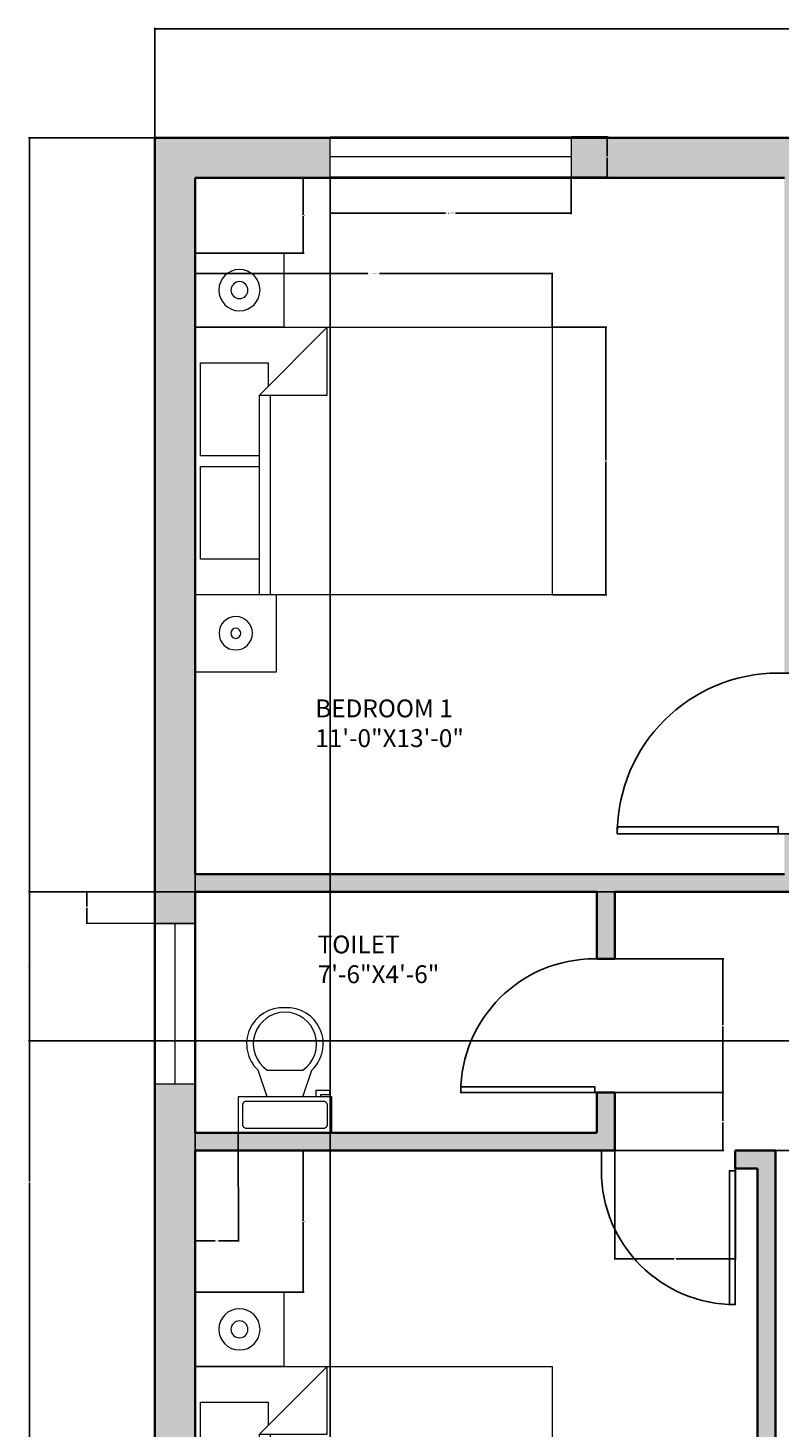
# Model space of a CAD drawing. Units: inches. Extents: x -29 to 443, y -589 to 39.
# Tile 3 of 5: x -29 to 139, y -275 to 39. Entities that reach past the tile are written whole.
import ezdxf

# ---------------------------------------------------------------- set-up
doc = ezdxf.new("R2010")
doc.units = ezdxf.units.IN
for name, color, linetype, lineweight in [('A-ANNO-DIMS', 2, 'Continuous', 18), ('A-AREA-IDEN', 7, 'Continuous', 18), ('A-DOOR', 3, 'Continuous', 25), ('A-FLOR-FIXT', 9, 'Continuous', 18), ('A-FURN', 9, 'Continuous', 18), ('A-GLAZ', 4, 'Continuous', 18), ('A-WALL', 7, 'Continuous', 35)]:
    doc.layers.add(name, color=color, linetype=linetype, lineweight=lineweight)
doc.layers.add('A-WALL-PATT', color=251, linetype='Continuous', lineweight=13, true_color=0x636466)
doc.styles.get("Standard").update_dxf_attribs({"font": 'arial.ttf'})
doc.dimstyles.get("Standard").update_dxf_attribs({"dimtxt": 0.18, "dimasz": 0.18, "dimexe": 0.18, "dimexo": 0.0625, "dimgap": 0.09, "dimtad": 0, "dimtih": 1, "dimtoh": 1, "dimdec": 4, "dimzin": 0, "dimdsep": 46, "dimtxsty": 'Standard', "dimcen": 0.09, "dimadec": 0, "dimazin": 0, "dimtfac": 1, "dimtdec": 4, "dimtofl": 0, "dimtmove": 0, "dimatfit": 3, "dimfxl": 1, "dimtolj": 1, "dimtzin": 0, "dimarcsym": 0})

# ---------------------------------------------------------------- blocks, each defined once
blk = doc.blocks.new('*U3')
for p, q in [((0, 0), (0, -6)), ((40, 0), (40, -6))]:
    blk.add_line(p, q)
blk.add_lwpolyline([(0, 0), (0, 40), (1.75, 40), (1.75, 0)], close=True)
blk.add_arc((0, 0), 40, 0, 90)
blk = doc.blocks.new('*U9')
for p, q in [((9.5, -6), (9.5, -2)), ((-10, -8.5), (-8, -8.5)), ((-10, -9.5), (-10, -8.5)), ((-8, -8.5), (-8, -8)), ((-7, -8), (-7, -9.5)), ((-4, -8), (-6, -14)), ((4, -8), (6, -14)), ((-7, -9.5), (-10, -9.5)), ((4, -14), (-4, -14))]:
    blk.add_line(p, q)
blk.add_lwpolyline([(10.5, -8), (10.5, 0), (-10.5, 0), (-10.5, -8)], close=True)
for points in [[(-9.5, -2), (-9.5, -6)], [(8.5, -1), (-8.5, -1)], [(-8.5, -7), (8.5, -7)]]:
    blk.add_lwpolyline(points)
for centre, radius, start, end in [((-8.625, -1.875), 0.8839, 81.8699, 188.1301), ((8.625, -1.875), 0.8839, 351.8699, 98.1301), ((-8.625, -6.125), 0.8839, 171.869898, 278.1301), ((8.625, -6.125), 0.8839, 261.8699, 8.1301), ((-0.4772, -19.9188), 8.0953, 133.01722, 273.38), ((0.0374, -19.8731), 7.127, 124.50543, 269.7), ((-0.0373, -19.8731), 7.127, 270.3, 55.4946), ((0.4773, -19.9188), 8.0953, 266.62, 46.9828)]:
    blk.add_arc(centre, radius, start, end)
blk = doc.blocks.new('Bed - Queen')
for p, q in [((0, -80.00003), (0, 0)), ((0, 0), (59.99999, 0)), ((59.99999, 0), (59.99999, -80.00003)), ((7.99999, -1.2), (28.79998, -1.2)), ((7.99999, -14.4), (7.99999, -1.2)), ((28.79998, -1.2), (28.79998, -14.4)), ((31.19999, -1.2), (51.99999, -1.2)), ((31.19999, -14.4), (31.19999, -1.2)), ((51.99999, -1.2), (51.99999, -16.4)), ((0, -14.4), (44.8, -14.4)), ((59.99999, -29.6), (44.8, -14.4)), ((44.8, -14.4), (44.8, -29.6)), ((44.8, -16.8), (0, -16.8)), ((51.99999, -16.4), (46.79936, -16.4)), ((44.8, -29.6), (59.99999, -29.6)), ((59.99999, -80.00003), (0, -80.00003))]:
    blk.add_line(p, q)
blk = doc.blocks.new('WIN-54IN')
blk.add_line((54, 4.5), (0, 4.5))
blk.add_lwpolyline([(0, 9), (54, 9), (54, 0), (0, 0)], close=True)
blk = doc.blocks.new('WIN-36IN')
blk.add_line((4.5, 36), (4.5, 0))
blk.add_lwpolyline([(0, 0), (0, 36), (9, 36), (9, 0)], close=True)
blk = doc.blocks.new('NIGHTSTAND-LARGE')
blk.add_lwpolyline([(19.87, 0), (19.87, 16.61), (0, 16.61), (0, 0)], close=True)
for radius in [4.62, 1.9]:
    blk.add_circle((9.93, 8.31), radius)
blk = doc.blocks.new('NIGHTSTAND-SMALL')
blk.add_lwpolyline([(18.21, 17.2), (18.21, 0), (0, 0), (0, 17.2)], close=True)
for radius in [3.74, 1.13]:
    blk.add_circle((9.11, 8.6), radius)
blk = doc.blocks.new('*D18')
at = {"layer": 'A-ANNO-DIMS', "color": 0, "lineweight": -2, "transparency": 16777216}
for p, q in [((38.66, 5.51), (38.66, -2.7)), ((92.66, 5.51), (92.66, -2.7)), ((38.84, -2.52), (64.55, -2.52)), ((92.48, -2.52), (66.78, -2.52))]:
    blk.add_line(p, q, dxfattribs=at)
at = {"layer": 'A-ANNO-DIMS', "color": 0, "transparency": 16777216}
for points in [[(38.84, -2.49), (38.84, -2.55), (38.66, -2.52)], [(92.48, -2.49), (92.48, -2.55), (92.66, -2.52)]]:
    blk.add_solid(points, dxfattribs=at)
at = {"layer": 'Defpoints', "color": 0, "transparency": 16777216}
for p in [(38.66, 5.58), (92.66, 5.58), (92.66, -2.52)]:
    blk.add_point(p, dxfattribs=at)
at = {"layer": 'A-ANNO-DIMS', "color": 0, "transparency": 16777216, "insert": (65.66, -2.52), "char_height": 0.18, "attachment_point": 5}
blk.add_mtext('\\A1;WINDOW 54 TYP.', dxfattribs=at)
blk = doc.blocks.new('*D19')
at = {"layer": 'A-ANNO-DIMS', "color": 0, "lineweight": -2, "transparency": 16777216}
for p, q in [((92.73, 14.58), (100.94, 14.58)), ((100.76, 14.4), (100.76, 10.26)), ((100.76, 5.76), (100.76, 9.89)), ((92.73, 5.58), (100.94, 5.58))]:
    blk.add_line(p, q, dxfattribs=at)
at = {"layer": 'A-ANNO-DIMS', "color": 0, "transparency": 16777216}
for points in [[(100.73, 14.4), (100.79, 14.4), (100.76, 14.58)], [(100.73, 5.76), (100.79, 5.76), (100.76, 5.58)]]:
    blk.add_solid(points, dxfattribs=at)
at = {"layer": 'Defpoints', "color": 0, "transparency": 16777216}
for p in [(92.66, 14.58), (100.76, 14.58), (92.66, 5.58)]:
    blk.add_point(p, dxfattribs=at)
at = {"layer": 'A-ANNO-DIMS', "color": 0, "transparency": 16777216, "insert": (100.76, 10.08), "char_height": 0.18, "attachment_point": 5}
blk.add_mtext('\\A1;9 TYP.', dxfattribs=at)
blk = doc.blocks.new('*D20')
at = {"layer": 'A-ANNO-DIMS', "color": 0, "lineweight": -2, "transparency": 16777216}
for p, q in [((8.44, -28.01), (8.44, -15.89)), ((8.62, -16.07), (47.13, -16.07)), ((88.26, -16.07), (49.74, -16.07)), ((88.44, -28.01), (88.44, -15.89))]:
    blk.add_line(p, q, dxfattribs=at)
at = {"layer": 'A-ANNO-DIMS', "color": 0, "transparency": 16777216}
for points in [[(8.62, -16.04), (8.62, -16.1), (8.44, -16.07)], [(88.26, -16.04), (88.26, -16.1), (88.44, -16.07)]]:
    blk.add_solid(points, dxfattribs=at)
at = {"layer": 'Defpoints', "color": 0, "transparency": 16777216}
for p in [(8.44, -16.07), (8.44, -28.07), (88.44, -28.07)]:
    blk.add_point(p, dxfattribs=at)
at = {"layer": 'A-ANNO-DIMS', "color": 0, "transparency": 16777216, "insert": (48.44, -16.07), "char_height": 0.18, "attachment_point": 5}
blk.add_mtext('\\A1;QUEEN BED 80 TYP.', dxfattribs=at)
blk = doc.blocks.new('*D21')
at = {"layer": 'A-ANNO-DIMS', "color": 0, "lineweight": -2, "transparency": 16777216}
for p, q in [((88.5, -28.07), (100.62, -28.07)), ((100.44, -28.25), (100.44, -57.89)), ((100.44, -87.89), (100.44, -58.26)), ((88.5, -88.07), (100.62, -88.07))]:
    blk.add_line(p, q, dxfattribs=at)
at = {"layer": 'A-ANNO-DIMS', "color": 0, "transparency": 16777216}
for points in [[(100.41, -28.25), (100.47, -28.25), (100.44, -28.07)], [(100.41, -87.89), (100.47, -87.89), (100.44, -88.07)]]:
    blk.add_solid(points, dxfattribs=at)
at = {"layer": 'Defpoints', "color": 0, "transparency": 16777216}
for p in [(88.44, -28.07), (100.44, -28.07), (88.44, -88.07)]:
    blk.add_point(p, dxfattribs=at)
at = {"layer": 'A-ANNO-DIMS', "color": 0, "transparency": 16777216, "insert": (100.44, -58.07), "char_height": 0.18, "attachment_point": 5}
blk.add_mtext('\\A1;60 TYP.', dxfattribs=at)
blk = doc.blocks.new('*D36')
at = {"layer": 'A-ANNO-DIMS', "color": 0, "lineweight": -2, "transparency": 16777216}
for p, q in [((-0.56, 14.45), (-0.56, 38.99)), ((-0.38, 38.81), (179.15, 38.81)), ((359.26, 38.81), (179.72, 38.81)), ((359.44, 14.45), (359.44, 38.99))]:
    blk.add_line(p, q, dxfattribs=at)
at = {"layer": 'A-ANNO-DIMS', "color": 0, "transparency": 16777216}
for points in [[(-0.38, 38.84), (-0.38, 38.78), (-0.56, 38.81)], [(359.26, 38.84), (359.26, 38.78), (359.44, 38.81)]]:
    blk.add_solid(points, dxfattribs=at)
at = {"layer": 'Defpoints', "color": 0, "transparency": 16777216}
for p in [(359.44, 38.81), (-0.56, 14.39), (359.44, 14.39)]:
    blk.add_point(p, dxfattribs=at)
at = {"layer": 'A-ANNO-DIMS', "color": 0, "transparency": 16777216, "insert": (179.44, 38.81), "char_height": 0.18, "attachment_point": 5}
blk.add_mtext('\\A1;360', dxfattribs=at)
blk = doc.blocks.new('*D37')
at = {"layer": 'A-ANNO-DIMS', "color": 0, "lineweight": -2, "transparency": 16777216}
for p, q in [((-0.63, 14.39), (-28.85, 14.39)), ((-28.67, 14.21), (-28.67, -219.43)), ((-28.67, -453.43), (-28.67, -219.8)), ((134.37, -453.61), (-28.85, -453.61))]:
    blk.add_line(p, q, dxfattribs=at)
at = {"layer": 'A-ANNO-DIMS', "color": 0, "transparency": 16777216}
for points in [[(-28.7, 14.21), (-28.64, 14.21), (-28.67, 14.39)], [(-28.7, -453.43), (-28.64, -453.43), (-28.67, -453.61)]]:
    blk.add_solid(points, dxfattribs=at)
at = {"layer": 'Defpoints', "color": 0, "transparency": 16777216}
for p in [(-0.56, 14.39), (-28.67, -453.61), (134.44, -453.61)]:
    blk.add_point(p, dxfattribs=at)
at = {"layer": 'A-ANNO-DIMS', "color": 0, "transparency": 16777216, "insert": (-28.67, -219.61), "char_height": 0.18, "attachment_point": 5}
blk.add_mtext('\\A1;468', dxfattribs=at)
blk = doc.blocks.new('*D38')
at = {"layer": 'A-ANNO-DIMS', "color": 0, "lineweight": -2, "transparency": 16777216}
for p, q in [((8.44, 5.32), (8.44, -492.89)), ((38.66, 5.51), (38.66, -492.89)), ((8.62, -492.71), (23.16, -492.71)), ((38.48, -492.71), (23.94, -492.71))]:
    blk.add_line(p, q, dxfattribs=at)
at = {"layer": 'A-ANNO-DIMS', "color": 0, "transparency": 16777216}
for points in [[(8.62, -492.68), (8.62, -492.74), (8.44, -492.71)], [(38.48, -492.68), (38.48, -492.74), (38.66, -492.71)]]:
    blk.add_solid(points, dxfattribs=at)
at = {"layer": 'Defpoints', "color": 0, "transparency": 16777216}
for p in [(8.44, 5.39), (38.66, 5.58), (8.44, -492.71)]:
    blk.add_point(p, dxfattribs=at)
at = {"layer": 'A-ANNO-DIMS', "color": 0, "transparency": 16777216, "insert": (23.55, -492.71), "char_height": 0.18, "attachment_point": 5}
blk.add_mtext('\\A1;30.23', dxfattribs=at)
blk = doc.blocks.new('*D41')
at = {"layer": 'A-ANNO-DIMS', "color": 0, "lineweight": -2, "transparency": 16777216}
for p, q in [((8.37, -154.61), (-15.97, -154.56)), ((-15.79, -154.74), (-15.8, -157.93)), ((-15.81, -161.48), (-15.8, -158.29)), ((8.36, -161.72), (-15.99, -161.66))]:
    blk.add_line(p, q, dxfattribs=at)
at = {"layer": 'A-ANNO-DIMS', "color": 0, "transparency": 16777216}
for points in [[(-15.82, -154.74), (-15.76, -154.74), (-15.79, -154.56)], [(-15.84, -161.48), (-15.78, -161.48), (-15.81, -161.66)]]:
    blk.add_solid(points, dxfattribs=at)
at = {"layer": 'Defpoints', "color": 0, "transparency": 16777216}
for p in [(-15.79, -154.56), (8.44, -154.61), (8.42, -161.72)]:
    blk.add_point(p, dxfattribs=at)
at = {"layer": 'A-ANNO-DIMS', "color": 0, "transparency": 16777216, "insert": (-15.8, -158.11), "char_height": 0.18, "attachment_point": 5}
blk.add_mtext('\\A1;7.106', dxfattribs=at)
blk = doc.blocks.new('*D59')
at = {"layer": 'A-ANNO-DIMS', "color": 0, "lineweight": -2, "transparency": 16777216}
for p, q in [((102.44, -212.68), (102.44, -237.02)), ((129.44, -212.68), (129.44, -237.02)), ((102.62, -236.84), (115.72, -236.84)), ((129.26, -236.84), (116.16, -236.84))]:
    blk.add_line(p, q, dxfattribs=at)
at = {"layer": 'A-ANNO-DIMS', "color": 0, "transparency": 16777216}
for points in [[(102.62, -236.81), (102.62, -236.87), (102.44, -236.84)], [(129.26, -236.81), (129.26, -236.87), (129.44, -236.84)]]:
    blk.add_solid(points, dxfattribs=at)
at = {"layer": 'Defpoints', "color": 0, "transparency": 16777216}
for p in [(102.44, -212.61), (129.44, -212.61), (102.44, -236.84)]:
    blk.add_point(p, dxfattribs=at)
at = {"layer": 'A-ANNO-DIMS', "color": 0, "transparency": 16777216, "insert": (115.94, -236.84), "char_height": 0.18, "attachment_point": 5}
blk.add_mtext('\\A1;27', dxfattribs=at)
blk = doc.blocks.new('*D64')
at = {"layer": 'A-ANNO-DIMS', "color": 0, "lineweight": -2, "transparency": 16777216}
for p, q in [((102.5, -169.61), (126.85, -169.61)), ((126.67, -169.79), (126.67, -184.43)), ((126.67, -199.43), (126.67, -184.8)), ((102.5, -199.61), (126.85, -199.61))]:
    blk.add_line(p, q, dxfattribs=at)
at = {"layer": 'A-ANNO-DIMS', "color": 0, "transparency": 16777216}
for points in [[(126.64, -169.79), (126.7, -169.79), (126.67, -169.61)], [(126.64, -199.43), (126.7, -199.43), (126.67, -199.61)]]:
    blk.add_solid(points, dxfattribs=at)
at = {"layer": 'Defpoints', "color": 0, "transparency": 16777216}
for p in [(102.44, -169.61), (102.44, -199.61), (126.67, -199.61)]:
    blk.add_point(p, dxfattribs=at)
at = {"layer": 'A-ANNO-DIMS', "color": 0, "transparency": 16777216, "insert": (126.67, -184.61), "char_height": 0.18, "attachment_point": 5}
blk.add_mtext('\\A1;30', dxfattribs=at)
blk = doc.blocks.new('*D65')
at = {"layer": 'A-ANNO-DIMS', "color": 0, "lineweight": -2, "transparency": 16777216}
for p, q in [((102.5, -199.61), (126.85, -199.61)), ((126.67, -199.79), (126.67, -205.93)), ((126.67, -212.43), (126.67, -206.3)), ((102.5, -212.61), (126.85, -212.61))]:
    blk.add_line(p, q, dxfattribs=at)
at = {"layer": 'A-ANNO-DIMS', "color": 0, "transparency": 16777216}
for points in [[(126.64, -199.79), (126.7, -199.79), (126.67, -199.61)], [(126.64, -212.43), (126.7, -212.43), (126.67, -212.61)]]:
    blk.add_solid(points, dxfattribs=at)
at = {"layer": 'Defpoints', "color": 0, "transparency": 16777216}
for p in [(102.44, -199.61), (102.44, -212.61), (126.67, -212.61)]:
    blk.add_point(p, dxfattribs=at)
at = {"layer": 'A-ANNO-DIMS', "color": 0, "transparency": 16777216, "insert": (126.67, -206.11), "char_height": 0.18, "attachment_point": 5}
blk.add_mtext('\\A1;13', dxfattribs=at)
blk = doc.blocks.new('*D66')
at = {"layer": 'A-ANNO-DIMS', "color": 0, "lineweight": -2, "transparency": 16777216}
for p, q in [((8.44, -208.68), (8.53, -233.02)), ((18.06, -208.64), (18.15, -232.99)), ((8.71, -232.84), (12.95, -232.83)), ((17.97, -232.81), (13.73, -232.82))]:
    blk.add_line(p, q, dxfattribs=at)
at = {"layer": 'A-ANNO-DIMS', "color": 0, "transparency": 16777216}
for points in [[(8.71, -232.81), (8.71, -232.87), (8.53, -232.84)], [(17.97, -232.78), (17.97, -232.84), (18.15, -232.81)]]:
    blk.add_solid(points, dxfattribs=at)
at = {"layer": 'Defpoints', "color": 0, "transparency": 16777216}
for p in [(8.44, -208.61), (18.06, -208.58), (8.53, -232.84)]:
    blk.add_point(p, dxfattribs=at)
at = {"layer": 'A-ANNO-DIMS', "color": 0, "transparency": 16777216, "insert": (13.34, -232.83), "char_height": 0.18, "attachment_point": 5}
blk.add_mtext('\\A1;9.624', dxfattribs=at)
blk = doc.blocks.new('*D75')
at = {"layer": 'A-ANNO-DIMS', "color": 0, "lineweight": -2, "transparency": 16777216}
for p, q in [((286.37, -154.61), (-28.85, -154.61)), ((-28.67, -154.79), (-28.67, -171.13)), ((-28.67, -187.82), (-28.67, -171.49)), ((265.22, -188), (-28.85, -188))]:
    blk.add_line(p, q, dxfattribs=at)
at = {"layer": 'A-ANNO-DIMS', "color": 0, "transparency": 16777216}
for points in [[(-28.7, -154.79), (-28.64, -154.79), (-28.67, -154.61)], [(-28.7, -187.82), (-28.64, -187.82), (-28.67, -188)]]:
    blk.add_solid(points, dxfattribs=at)
at = {"layer": 'Defpoints', "color": 0, "transparency": 16777216}
for p in [(-28.67, -154.61), (286.44, -154.61), (265.28, -188)]:
    blk.add_point(p, dxfattribs=at)
at = {"layer": 'A-ANNO-DIMS', "color": 0, "transparency": 16777216, "insert": (-28.67, -171.31), "char_height": 0.18, "attachment_point": 5}
blk.add_mtext('\\A1;33.39', dxfattribs=at)
blk = doc.blocks.new('*D79')
at = {"layer": 'A-ANNO-DIMS', "color": 0, "lineweight": -2, "transparency": 16777216}
for p, q in [((8.5, 5.39), (32.85, 5.39)), ((32.67, 5.21), (32.67, -2.86)), ((32.67, -11.28), (32.67, -3.22)), ((8.5, -11.46), (32.85, -11.46))]:
    blk.add_line(p, q, dxfattribs=at)
at = {"layer": 'A-ANNO-DIMS', "color": 0, "transparency": 16777216}
for points in [[(32.64, 5.21), (32.7, 5.21), (32.67, 5.39)], [(32.64, -11.28), (32.7, -11.28), (32.67, -11.46)]]:
    blk.add_solid(points, dxfattribs=at)
at = {"layer": 'Defpoints', "color": 0, "transparency": 16777216}
for p in [(8.44, 5.39), (8.44, -11.46), (32.67, -11.46)]:
    blk.add_point(p, dxfattribs=at)
at = {"layer": 'A-ANNO-DIMS', "color": 0, "transparency": 16777216, "insert": (32.67, -3.04), "char_height": 0.18, "attachment_point": 5}
blk.add_mtext('\\A1;16.847', dxfattribs=at)
blk = doc.blocks.new('*D81')
at = {"layer": 'A-ANNO-DIMS', "color": 0, "lineweight": -2, "transparency": 16777216}
for p, q in [((8.5, -212.61), (32.85, -212.61)), ((32.67, -212.79), (32.67, -228.31)), ((32.67, -244.18), (32.67, -228.67)), ((8.5, -244.36), (32.85, -244.36))]:
    blk.add_line(p, q, dxfattribs=at)
at = {"layer": 'A-ANNO-DIMS', "color": 0, "transparency": 16777216}
for points in [[(32.64, -212.79), (32.7, -212.79), (32.67, -212.61)], [(32.64, -244.18), (32.7, -244.18), (32.67, -244.36)]]:
    blk.add_solid(points, dxfattribs=at)
at = {"layer": 'Defpoints', "color": 0, "transparency": 16777216}
for p in [(8.44, -212.61), (8.44, -244.36), (32.67, -244.36)]:
    blk.add_point(p, dxfattribs=at)
at = {"layer": 'A-ANNO-DIMS', "color": 0, "transparency": 16777216, "insert": (32.67, -228.49), "char_height": 0.18, "attachment_point": 5}
blk.add_mtext('\\A1;31.75', dxfattribs=at)
blk = doc.blocks.new('*D82')
at = {"layer": 'A-ANNO-DIMS', "color": 0, "lineweight": -2, "transparency": 16777216}
for p, q in [((138.5, -212.61), (383.85, -212.61)), ((383.67, -212.79), (383.67, -231.59)), ((383.67, -250.74), (383.67, -231.95)), ((152.45, -250.92), (383.85, -250.92))]:
    blk.add_line(p, q, dxfattribs=at)
at = {"layer": 'A-ANNO-DIMS', "color": 0, "transparency": 16777216}
for points in [[(383.64, -212.79), (383.7, -212.79), (383.67, -212.61)], [(383.64, -250.74), (383.7, -250.74), (383.67, -250.92)]]:
    blk.add_solid(points, dxfattribs=at)
at = {"layer": 'Defpoints', "color": 0, "transparency": 16777216}
for p in [(138.44, -212.61), (152.39, -250.92), (383.67, -250.92)]:
    blk.add_point(p, dxfattribs=at)
at = {"layer": 'A-ANNO-DIMS', "color": 0, "transparency": 16777216, "insert": (383.67, -231.77), "char_height": 0.18, "attachment_point": 5}
blk.add_mtext('\\A1;38.31', dxfattribs=at)

msp = doc.modelspace()

# ---------------------------------------------------------------- hatches: boundary and pattern name
at = {"layer": 'A-WALL-PATT'}
h = msp.add_hatch(color=256, dxfattribs=at)
h.dxf.hatch_style = 1
h.paths.add_polyline_path([(8.4359, 5.3851), (38.6638, 5.3851), (38.6638, 14.3851), (-0.5641, 14.3851), (-0.5641, -161.7206), (8.4359, -161.7206), (8.4359, -154.6149), (98.4359, -154.6149), (98.4359, -169.6149), (102.4359, -169.6149), (102.4359, -154.6149), (144.4359, -154.6149), (144.4359, -141.6149), (140.4359, -141.6149), (140.4359, -150.6149), (8.4359, -150.6149)])
h.paths.add_polyline_path([(153.762, 14.3851), (92.6638, 14.3851), (92.6638, 5.3851), (140.4359, 5.3851), (140.4359, -105.5868), (144.4359, -105.5868), (144.4359, -94.6149), (153.4359, -94.6149), (153.4359, -90.6149), (144.4359, -90.6149), (144.4359, 5.3851), (153.762, 5.3851)])
h.paths.add_polyline_path([(264.576, 14.3851), (189.762, 14.3851), (189.762, 5.3851), (204.4359, 5.3851), (204.4359, -40.0486, -0.11439146), (204.5889, -40.7086), (204.5889, -67.7086, -0.11439146), (204.4359, -68.3685), (204.4359, -90.6149), (183.4359, -90.6149), (183.4359, -94.6149), (204.4359, -94.6149), (204.4359, -108.4622), (208.4359, -108.4622), (208.4359, 5.3851), (264.576, 5.3851)])
h.paths.add_polyline_path([(359.4359, 14.3851), (318.576, 14.3851), (318.576, 5.3851), (350.4359, 5.3851), (350.4359, -150.6149), (208.4359, -150.6149), (208.4359, -144.6149), (204.4359, -144.6149), (204.4359, -154.6149), (286.4359, -154.6149), (286.4359, -169.4775), (290.4359, -169.4775), (290.4359, -154.6149), (359.4359, -154.6149)])
h.paths.add_polyline_path([(8.4359, -212.6149), (98.4359, -212.6149), (102.4359, -212.6149), (102.4359, -199.6149), (98.4359, -199.6149), (98.4359, -208.6149), (8.4359, -208.6149), (8.4359, -197.7206), (-0.5641, -197.7206), (-0.5641, -417.6149), (114.4359, -417.6149), (114.4359, -354.6149), (134.4359, -354.6149), (134.4359, -453.6149), (147.4359, -453.6149), (147.4359, -444.6149), (138.4359, -444.6149), (138.4359, -212.6149), (129.4359, -212.6149), (129.4359, -216.6149), (134.4359, -216.6149), (134.4359, -350.6149), (110.4359, -350.6149), (110.4359, -377.2063, -0.30395766), (111.1497, -378.2719, -0.30395766), (110.4359, -379.3376), (110.4359, -408.6149), (8.4359, -408.6149)])
h.paths.add_polyline_path([(265.0252, -444.6149), (230.4359, -444.6149), (230.4359, -396.6149), (246.223, -396.6149), (246.223, -392.6149), (230.4359, -392.6149), (230.4359, -302.6149), (245.4886, -302.6149), (245.4886, -298.6149), (226.4359, -298.6149), (226.4359, -444.6149), (189.4359, -444.6149), (189.4359, -453.6149), (226.4359, -453.6149), (265.0252, -453.6149)])
h.paths.add_polyline_path([(359.4359, -417.6149), (359.4359, -377.3771), (350.4359, -377.3771), (350.4359, -392.6149), (276.3235, -392.6149), (276.3235, -396.6149), (350.4359, -396.6149), (350.4359, -408.6149), (350.4359, -444.6149), (319.0252, -444.6149), (319.0252, -453.6149), (359.4359, -453.6149)])
h.paths.add_polyline_path([(359.4359, -298.6149), (290.4359, -298.6149), (290.4359, -289.6207), (286.4359, -289.6207), (286.4359, -298.6149), (277.8355, -298.6149), (277.8355, -302.6149), (350.4359, -302.6149), (350.4359, -323.3771), (359.4359, -323.3771)])
h.paths.add_polyline_path([(290.4359, -226.7916), (286.4359, -226.7916), (286.4359, -253.468), (290.4359, -253.468)])

# ---------------------------------------------------------------- linework, layer by layer
at = {"layer": 'A-WALL'}
for p, q in [((-0.5641, -417.6149), (-0.5641, 14.3851)), ((-0.5641, 14.3851), (359.4359, 14.3851)), ((8.4359, 5.3851), (140.4359, 5.3851)), ((8.4359, -150.6149), (8.4359, 5.3851)), ((8.4359, -150.6149), (140.4359, -150.6149)), ((8.4359, -154.6149), (98.4359, -154.6149)), ((8.4359, -208.6149), (8.4359, -154.6149)), ((98.4359, -169.6182), (98.4359, -154.6149)), ((102.4359, -154.6149), (144.4359, -154.6149)), ((102.4359, -169.6182), (102.4359, -154.6149)), ((98.4359, -169.6149), (102.4359, -169.6149)), ((98.4359, -208.6149), (98.4359, -199.6149)), ((98.4359, -208.6149), (98.4359, -199.6149)), ((98.4359, -199.6149), (102.4359, -199.6149)), ((102.4359, -212.6149), (102.4359, -199.6149)), ((8.4359, -208.6149), (98.4359, -208.6149)), ((8.4359, -212.6149), (98.4359, -212.6149)), ((8.4359, -408.6149), (8.4359, -212.6149)), ((98.4359, -212.6149), (102.4359, -212.6149)), ((138.4359, -212.6149), (129.4359, -212.6149)), ((129.4359, -212.6149), (129.4359, -216.6149)), ((138.4359, -212.6149), (134.4359, -212.6149)), ((138.4359, -444.6149), (138.4359, -212.6149)), ((129.4359, -216.6149), (134.4359, -216.6149)), ((134.4359, -350.6149), (134.4359, -216.6149))]:
    msp.add_line(p, q, dxfattribs=at)

# ---------------------------------------------------------------- block references
at = {"layer": 'A-DOOR'}
for p, xscale, yscale, zscale, rotation in [((139.0317, -141.6149), 0.9007031816265564, 0.9007031816265564, 0.9007031816265564, 90), ((97.9364, -199.6149), 0.7499177992314163, 0.7499177992314163, 0.7499177992314163, 90), ((129.4359, -217.1144), 0.7499177992314163, 0.7499177992314163, 0.7499177992314163, 180)]:
    msp.add_blockref('*U3', p, dxfattribs=dict(at, xscale=xscale, yscale=yscale, zscale=zscale, rotation=rotation))
at = {"layer": 'A-FLOR-FIXT', "rotation": 180}
msp.add_blockref('*U9', (28.5602, -208.5779), dxfattribs=at)
at = {"layer": 'A-FURN', "extrusion": (0, 0, -1), "zscale": -1}
for name, p in [('NIGHTSTAND-LARGE', (-28.3059, -28.073)), ('NIGHTSTAND-SMALL', (-26.6499, -105.269)), ('NIGHTSTAND-LARGE', (-28.3059, -260.9742))]:
    msp.add_blockref(name, p, dxfattribs=at)
at = {"layer": 'A-FURN', "rotation": 90}
for p in [(8.4359, -88.0734), (8.4359, -320.9746)]:
    msp.add_blockref('Bed - Queen', p, dxfattribs=at)
at = {"layer": 'A-GLAZ'}
for name, p in [('WIN-54IN', (38.664, 5.576)), ('WIN-36IN', (-0.581, -197.721))]:
    msp.add_blockref(name, p, dxfattribs=at)

# ---------------------------------------------------------------- texts
at = {"layer": 'A-AREA-IDEN', "char_height": 4, "attachment_point": 1}
for s, width, insert in [('BEDROOM 1\\P11\'-0"X13\'-0"', 58.755484, (35.3499, -111.5006)), ('TOILET\\P7\'-6"X4\'-6"', 43.723497, (35.9008, -164.408))]:
    msp.add_mtext_dynamic_manual_height_columns(s, width=width, gutter_width=12.5, heights=[0], dxfattribs=dict(at, insert=insert))

# ---------------------------------------------------------------- dimensions: what is measured, and where the dimension line sits
at = {"layer": 'A-ANNO-DIMS'}
for base, p1, p2, override, picture, middle in [((359.4359, 38.8064), (-0.5641, 14.3851), (359.4359, 14.3851), {"dimdec": 0, "dimlfac": 1, "dimrnd": 0, "dimzin": 0, "dimdsep": 46, "dimlunit": 2}, '*D36', (179.4359, 38.8064)), ((8.4359, -492.7145), (38.6638, 5.5764), (8.4359, 5.3851), {"dimdec": 2, "dimlfac": 1, "dimrnd": 0, "dimzin": 0, "dimdsep": 46, "dimlunit": 2}, '*D38', (23.5499, -492.7145))]:
    dim = msp.add_linear_dim(base=base, p1=p1, p2=p2, dimstyle='Standard', override=override, dxfattribs=at)
    dim.commit()
    dim.dimension.update_dxf_attribs({"geometry": picture, "text_midpoint": middle})
for base, p1, p2, angle, override, picture, middle in [((-28.6698, -453.6149), (-0.5641, 14.3851), (134.4359, -453.6149), 90, {"dimdec": 0, "dimlfac": 1, "dimrnd": 0, "dimzin": 0, "dimdsep": 46, "dimlunit": 2}, '*D37', (-28.6698, -219.6149)), ((32.6659, -11.4618), (8.4359, 5.3851), (8.4359, -11.4618), 270, {"dimdec": 3, "dimlfac": 1, "dimrnd": 0, "dimzin": 0, "dimdsep": 46, "dimlunit": 2}, '*D79', (32.6659, -3.0384)), ((-28.6698, -154.6149), (265.284, -188.0033), (286.4359, -154.6149), 90, {"dimdec": 2, "dimlfac": 1, "dimrnd": 0, "dimzin": 0, "dimdsep": 46, "dimlunit": 2}, '*D75', (-28.6698, -171.3091)), ((-15.794, -154.5576), (8.4191, -161.7206), (8.4359, -154.6149), 89.86446, {"dimdec": 3, "dimlfac": 1, "dimrnd": 0, "dimzin": 0, "dimdsep": 46, "dimlunit": 2}, '*D41', (-15.8024, -158.1104)), ((126.6659, -199.6149), (102.4359, -169.6149), (102.4359, -199.6149), 270, {"dimdec": 0, "dimlfac": 1, "dimrnd": 0, "dimzin": 0, "dimdsep": 46, "dimlunit": 2}, '*D64', (126.6659, -184.6149)), ((126.6659, -212.6149), (102.4359, -199.6149), (102.4359, -212.6149), 270, {"dimdec": 0, "dimlfac": 1, "dimrnd": 0, "dimzin": 0, "dimdsep": 46, "dimlunit": 2}, '*D65', (126.6659, -206.1149)), ((8.5293, -232.8447), (18.0602, -208.5779), (8.4359, -208.6149), 180.22065, {"dimdec": 3, "dimlfac": 1, "dimrnd": 0, "dimzin": 0, "dimdsep": 46, "dimlunit": 2}, '*D66', (13.3414, -232.8262)), ((32.6659, -244.363), (8.4359, -212.6149), (8.4359, -244.363), 270, {"dimdec": 2, "dimlfac": 1, "dimrnd": 0, "dimzin": 0, "dimdsep": 46, "dimlunit": 2}, '*D81', (32.6659, -228.489)), ((102.4359, -236.8449), (129.4359, -212.6149), (102.4359, -212.6149), 180, {"dimdec": 0, "dimlfac": 1, "dimrnd": 0, "dimzin": 0, "dimdsep": 46, "dimlunit": 2}, '*D59', (115.9359, -236.8449)), ((383.6659, -250.9234), (138.4359, -212.6149), (152.3905, -250.9234), 90, {"dimdec": 2, "dimlfac": 1, "dimrnd": 0, "dimzin": 0, "dimdsep": 46, "dimlunit": 2}, '*D82', (383.6659, -231.7692))]:
    dim = msp.add_linear_dim(base=base, p1=p1, p2=p2, angle=angle, dimstyle='Standard', override=override, dxfattribs=at)
    dim.commit()
    dim.dimension.update_dxf_attribs({"geometry": picture, "text_midpoint": middle})
for base, p1, p2, angle, text, picture, middle in [((100.7638, 14.5764), (92.6638, 5.5764), (92.6638, 14.5764), 90, '<> TYP.', '*D19', (100.7638, 10.0764)), ((8.4359, -16.0734), (88.436, -28.0734), (8.4359, -28.0734), 180, 'QUEEN BED <> TYP.', '*D20', (48.436, -16.0734)), ((100.436, -28.0734), (88.436, -88.0734), (88.436, -28.0734), 90, '<> TYP.', '*D21', (100.436, -58.0734))]:
    dim = msp.add_linear_dim(base=base, p1=p1, p2=p2, angle=angle, text=text, dimstyle='Standard', override={"dimdec": 0, "dimlfac": 1, "dimrnd": 0, "dimzin": 0, "dimdsep": 46, "dimlunit": 2}, dxfattribs=at)
    dim.commit()
    dim.dimension.update_dxf_attribs({"geometry": picture, "text_midpoint": middle})
dim = msp.add_linear_dim(base=(92.6638, -2.5236), p1=(38.6638, 5.5764), p2=(92.6638, 5.5764), text='WINDOW <> TYP.', dimstyle='Standard', override={"dimdec": 0, "dimlfac": 1, "dimrnd": 0, "dimzin": 0, "dimdsep": 46, "dimlunit": 2}, dxfattribs=at)
dim.commit()
dim.dimension.update_dxf_attribs({"geometry": '*D18', "text_midpoint": (65.6638, -2.5236)})

doc.saveas('drawing.dxf')
